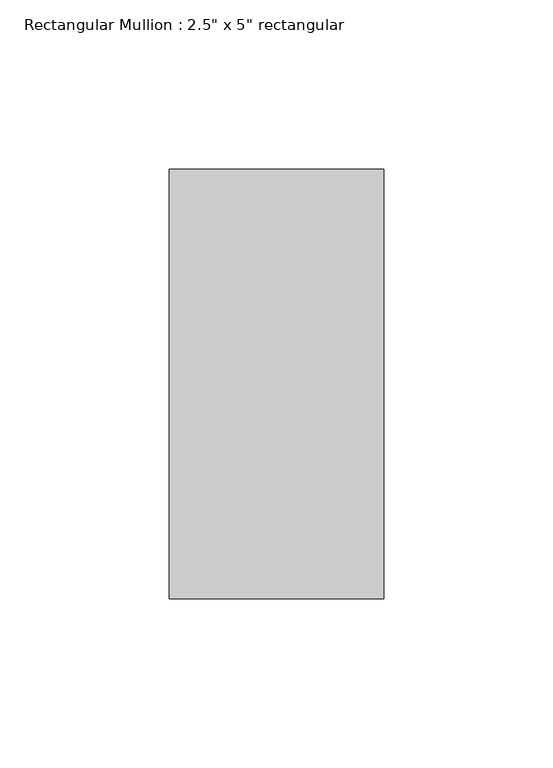
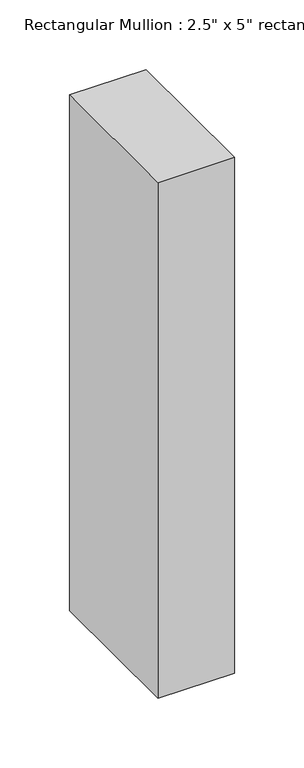
"""IFC4 building model written with IfcOpenShell, lengths in millimetres: member geometry."""

from ifc_helpers import new_model, si_unit, frame, origin, place, context, project, spatial, polyline, outline, extrude, source, transform, mapped, element, save


def member_2fb86761(model_context):
    return source(origin(), model_context, "Body", "SweptSolid", [
        extrude(outline(polyline([(0.0, 63.5), (0.0, -63.5), (-63.5, -63.5), (-63.5, 63.5), (0.0, 63.5)])), frame((0.0, 0.0, -452.0931105), z_axis=(0.0, 0.0, 1.0), x_axis=(1.0, 0.0, 0.0)), (0.0, 0.0, 1.0), 452.0931105),
    ])


if __name__ == "__main__":
    model = new_model("IFC4")
    model_context = context("Model", 3, world=origin())
    ifc_project = project(units=[si_unit("LENGTHUNIT", "METRE", prefix="MILLI")], contexts=[model_context])
    site = spatial("IfcSite", under=ifc_project)
    building = spatial("IfcBuilding", under=site)
    placement = place(None, origin())
    member_shape = member_2fb86761(model_context)
    element("IfcMember", 1, ObjectType="Rectangular Mullion : 2.5\" x 5\" rectangular", at=placement, inside=building, context=model_context, shape_type="MappedRepresentation", body=[
        mapped(member_shape, transform((0.0, 0.0, 0.0), x_axis=(1.0, 0.0, 0.0), y_axis=(0.0, 1.0, 0.0), z_axis=(0.0, 0.0, 1.0))),
    ])
    save(model, "model.ifc")

# Revit data of these elements
# Type "Rectangular Mullion : 2.5\" x 5\" rectangular"
#   built-in parameter 1007304 = 0.416667 (stored number, unit not read)
#   built-in parameter 1007301 = 0.104167 (stored number, unit not read)
#   built-in parameter 1007300 = 0.104167 (stored number, unit not read)
# Element 1 (IfcMember, "Rectangular Mullion : 2.5\" x 5\" rectangular")
#   Materials on its faces: "Aluminum"
# Materials
#   "Aluminum": class "Metal", colour RGB 247 247 247, transparency 0, Description = "Aluminum 6061", Cost = 0
